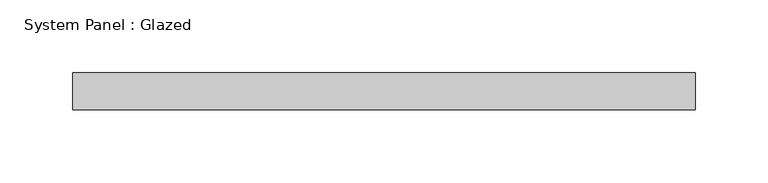
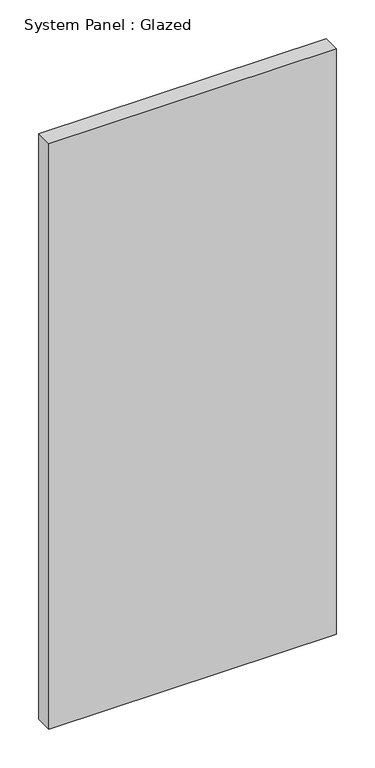
"""IFC4 building model written with IfcOpenShell, lengths in millimetres: plate geometry, System Panel : Glazed."""

from ifc_helpers import new_model, si_unit, origin, origin_with_axes, place, context, project, spatial, polyline, outline, extrude, source, transform, mapped, element, save


def system_panel_glazed_9bb7629d(model_context):
    return source(origin(), model_context, "Body", "SweptSolid", [
        extrude(outline(polyline([(213.7833333, 19.05), (-213.7833333, 19.05), (-213.7833333, 44.45), (213.7833333, 44.45), (213.7833333, 19.05)])), origin_with_axes(), (0.0, 0.0, 1.0), 920.75),
    ])


if __name__ == "__main__":
    model = new_model("IFC4")
    model_context = context("Model", 3, world=origin())
    ifc_project = project(units=[si_unit("LENGTHUNIT", "METRE", prefix="MILLI")], contexts=[model_context])
    site = spatial("IfcSite", under=ifc_project)
    building = spatial("IfcBuilding", under=site)
    placement = place(None, origin())
    system_panel_glazed_shape = system_panel_glazed_9bb7629d(model_context)
    element("IfcPlate", 1, ObjectType="System Panel : Glazed", at=placement, inside=building, context=model_context, shape_type="MappedRepresentation", body=[
        mapped(system_panel_glazed_shape, transform((0.0, 0.0, 0.0), x_axis=(1.0, 0.0, 0.0), y_axis=(0.0, 1.0, 0.0), z_axis=(0.0, 0.0, 1.0))),
    ])
    save(model, "model.ifc")

# Revit data of these elements
# Type "System Panel : Glazed"
#   Construction Type Id = "GSP4R"
#   Analytic Construction = "1/8 in Pilkington single glazing"
#   Visual Light Transmittance = 0.9
#   Solar Heat Gain Coefficient = 0.86
#   Heat Transfer Coefficient (U) = 1.18115 BTU/(h·ft²·°F)
#   Define Thermal Properties by = 1
# Element 1 (IfcPlate, "System Panel : Glazed")
#   Materials on its faces: "Glass"
# Materials
#   "Glass": class "Glass", colour RGB 0 128 192, transparency 0.75, Description = "Soda Lime Glass", Cost = 0
